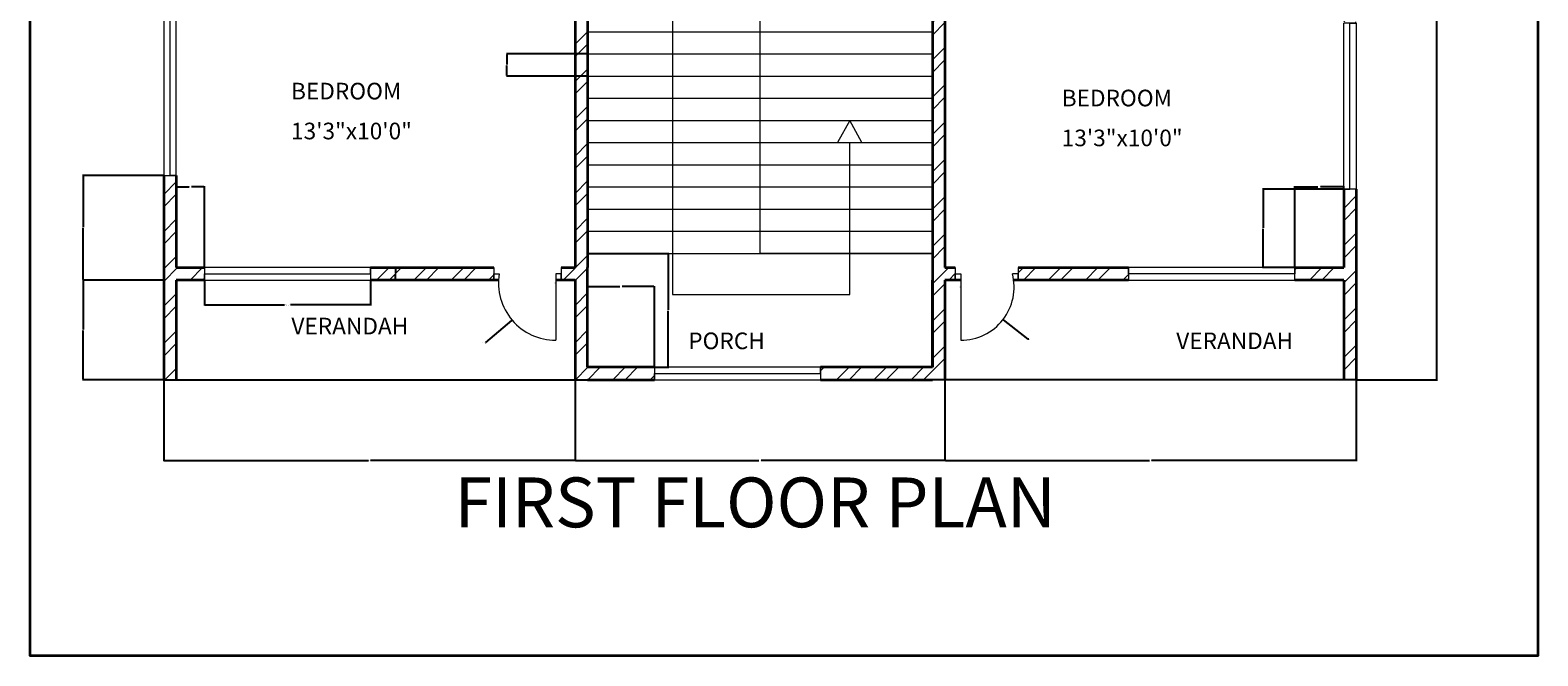
# Model space of a CAD drawing. Units: inches. Extents: x 2271 to 2815, y 1169 to 1838.
# Tile 1 of 4: x 2271 to 2815, y 1169 to 1395. Entities that reach past the tile are written whole.
import ezdxf

# ---------------------------------------------------------------- set-up
doc = ezdxf.new("R2010")
doc.units = ezdxf.units.IN
for name, color, linetype, lineweight in [('A-ANNO-DIMS', 2, 'Continuous', 18), ('A-ANNO-SYMB', 101, 'Continuous', 13), ('A-ANNO-TITL', 151, 'Continuous', 35), ('A-ANNO-TTLB', 7, 'Continuous', 35), ('A-AREA-IDEN', 7, 'Continuous', 18), ('A-DOOR', 11, 'Continuous', 18), ('A-FLOR-EDGE', 7, 'Continuous', 25), ('A-FLOR-STRS', 101, 'Continuous', 18), ('A-GLAZ', 181, 'Continuous', 18), ('A-WALL', 7, 'Continuous', 35)]:
    doc.layers.add(name, color=color, linetype=linetype, lineweight=lineweight)
doc.layers.add('A-WALL-PATT', color=9, linetype='Continuous', lineweight=13, true_color=0xafd9aa)
doc.styles.get("Standard").update_dxf_attribs({"font": 'arial.ttf'})
doc.dimstyles.get("Standard").update_dxf_attribs({"dimtxt": 0.18, "dimasz": 0.18, "dimexe": 0.18, "dimexo": 0.0625, "dimgap": 0.09, "dimtad": 0, "dimtih": 1, "dimtoh": 1, "dimdec": 4, "dimzin": 0, "dimdsep": 46, "dimtxsty": 'Standard', "dimcen": 0.09, "dimadec": 0, "dimazin": 0, "dimtfac": 1, "dimtdec": 4, "dimtofl": 0, "dimtmove": 0, "dimatfit": 3, "dimfxl": 1, "dimtolj": 1, "dimtzin": 0, "dimarcsym": 0})

# ---------------------------------------------------------------- blocks, each defined once
blk = doc.blocks.new('WIN-60IN')
for p, q in [((0, 4.5), (0, 0)), ((60, 4.5), (0, 4.5)), ((0, 0), (0, 2.25)), ((0, 2.25), (60, 2.25)), ((0, 0), (60, 0)), ((60, 2.25), (60, 4.5)), ((60, 4.5), (60, 0))]:
    blk.add_line(p, q)
blk = doc.blocks.new('*D3')
at = {"layer": 'A-ANNO-DIMS', "color": 0, "lineweight": -2, "transparency": 16777216}
for p, q in [((2333.47, 1304.47), (2333.47, 1295.35)), ((2393.47, 1304.47), (2393.47, 1295.35)), ((2333.65, 1295.53), (2362.35, 1295.53)), ((2393.29, 1295.53), (2364.58, 1295.53))]:
    blk.add_line(p, q, dxfattribs=at)
at = {"layer": 'A-ANNO-DIMS', "color": 0, "transparency": 16777216}
for points in [[(2333.65, 1295.56), (2333.65, 1295.5), (2333.47, 1295.53)], [(2393.29, 1295.56), (2393.29, 1295.5), (2393.47, 1295.53)]]:
    blk.add_solid(points, dxfattribs=at)
at = {"layer": 'Defpoints', "color": 0, "transparency": 16777216}
for p in [(2333.47, 1304.53), (2393.47, 1304.53), (2393.47, 1295.53)]:
    blk.add_point(p, dxfattribs=at)
at = {"layer": 'A-ANNO-DIMS', "color": 0, "transparency": 16777216, "insert": (2363.47, 1295.53), "char_height": 0.18, "attachment_point": 5}
blk.add_mtext('\\A1;WINDOW 60 TYP.', dxfattribs=at)
blk = doc.blocks.new('*D4')
at = {"layer": 'A-ANNO-DIMS', "color": 0, "lineweight": -2, "transparency": 16777216}
for p, q in [((2393.53, 1309.03), (2402.65, 1309.03)), ((2402.47, 1308.85), (2402.47, 1306.96)), ((2402.47, 1304.71), (2402.47, 1306.6)), ((2393.53, 1304.53), (2402.65, 1304.53))]:
    blk.add_line(p, q, dxfattribs=at)
at = {"layer": 'A-ANNO-DIMS', "color": 0, "transparency": 16777216}
for points in [[(2402.44, 1308.85), (2402.5, 1308.85), (2402.47, 1309.03)], [(2402.44, 1304.71), (2402.5, 1304.71), (2402.47, 1304.53)]]:
    blk.add_solid(points, dxfattribs=at)
at = {"layer": 'Defpoints', "color": 0, "transparency": 16777216}
for p in [(2393.47, 1309.03), (2402.47, 1309.03), (2393.47, 1304.53)]:
    blk.add_point(p, dxfattribs=at)
at = {"layer": 'A-ANNO-DIMS', "color": 0, "transparency": 16777216, "insert": (2402.47, 1306.78), "char_height": 0.18, "attachment_point": 5}
blk.add_mtext('\\A1;5 TYP.', dxfattribs=at)
blk = doc.blocks.new('*D8')
at = {"layer": 'A-ANNO-DIMS', "color": 0, "lineweight": -2, "transparency": 16777216}
for p, q in [((2749.36, 1787.53), (2778.63, 1787.53)), ((2778.45, 1787.35), (2778.45, 1528.21)), ((2778.45, 1268.71), (2778.45, 1527.85)), ((2749.36, 1268.53), (2778.63, 1268.53))]:
    blk.add_line(p, q, dxfattribs=at)
at = {"layer": 'A-ANNO-DIMS', "color": 0, "transparency": 16777216}
for points in [[(2778.42, 1787.35), (2778.48, 1787.35), (2778.45, 1787.53)], [(2778.42, 1268.71), (2778.48, 1268.71), (2778.45, 1268.53)]]:
    blk.add_solid(points, dxfattribs=at)
at = {"layer": 'Defpoints', "color": 0, "transparency": 16777216}
for p in [(2749.3, 1787.53), (2778.45, 1787.53), (2749.3, 1268.53)]:
    blk.add_point(p, dxfattribs=at)
at = {"layer": 'A-ANNO-DIMS', "color": 0, "transparency": 16777216, "insert": (2778.45, 1528.03), "char_height": 0.18, "attachment_point": 5}
blk.add_mtext('\\A1;519', dxfattribs=at)
blk = doc.blocks.new('*D9')
at = {"layer": 'A-ANNO-DIMS', "color": 0, "lineweight": -2, "transparency": 16777216}
for p, q in [((2318.8, 1268.47), (2318.8, 1239.2)), ((2467.3, 1268.47), (2467.3, 1239.2)), ((2318.98, 1239.38), (2392.66, 1239.38)), ((2467.12, 1239.38), (2393.44, 1239.38))]:
    blk.add_line(p, q, dxfattribs=at)
at = {"layer": 'A-ANNO-DIMS', "color": 0, "transparency": 16777216}
for points in [[(2318.98, 1239.41), (2318.98, 1239.35), (2318.8, 1239.38)], [(2467.12, 1239.41), (2467.12, 1239.35), (2467.3, 1239.38)]]:
    blk.add_solid(points, dxfattribs=at)
at = {"layer": 'Defpoints', "color": 0, "transparency": 16777216}
for p in [(2318.8, 1268.53), (2467.3, 1268.53), (2467.3, 1239.38)]:
    blk.add_point(p, dxfattribs=at)
at = {"layer": 'A-ANNO-DIMS', "color": 0, "transparency": 16777216, "insert": (2393.05, 1239.38), "char_height": 0.18, "attachment_point": 5}
blk.add_mtext('\\A1;148.5', dxfattribs=at)
blk = doc.blocks.new('*D10')
at = {"layer": 'A-ANNO-DIMS', "color": 0, "lineweight": -2, "transparency": 16777216}
for p, q in [((2467.3, 1268.47), (2467.3, 1239.2)), ((2600.8, 1268.47), (2600.8, 1239.2)), ((2467.48, 1239.38), (2533.66, 1239.38)), ((2600.62, 1239.38), (2534.44, 1239.38))]:
    blk.add_line(p, q, dxfattribs=at)
at = {"layer": 'A-ANNO-DIMS', "color": 0, "transparency": 16777216}
for points in [[(2467.48, 1239.41), (2467.48, 1239.35), (2467.3, 1239.38)], [(2600.62, 1239.41), (2600.62, 1239.35), (2600.8, 1239.38)]]:
    blk.add_solid(points, dxfattribs=at)
at = {"layer": 'Defpoints', "color": 0, "transparency": 16777216}
for p in [(2467.3, 1268.53), (2600.8, 1268.53), (2600.8, 1239.38)]:
    blk.add_point(p, dxfattribs=at)
at = {"layer": 'A-ANNO-DIMS', "color": 0, "transparency": 16777216, "insert": (2534.05, 1239.38), "char_height": 0.18, "attachment_point": 5}
blk.add_mtext('\\A1;133.5', dxfattribs=at)
blk = doc.blocks.new('*D11')
at = {"layer": 'A-ANNO-DIMS', "color": 0, "lineweight": -2, "transparency": 16777216}
for p, q in [((2600.8, 1268.47), (2600.8, 1239.2)), ((2749.3, 1268.47), (2749.3, 1239.2)), ((2600.98, 1239.38), (2674.66, 1239.38)), ((2749.12, 1239.38), (2675.44, 1239.38))]:
    blk.add_line(p, q, dxfattribs=at)
at = {"layer": 'A-ANNO-DIMS', "color": 0, "transparency": 16777216}
for points in [[(2600.98, 1239.41), (2600.98, 1239.35), (2600.8, 1239.38)], [(2749.12, 1239.41), (2749.12, 1239.35), (2749.3, 1239.38)]]:
    blk.add_solid(points, dxfattribs=at)
at = {"layer": 'Defpoints', "color": 0, "transparency": 16777216}
for p in [(2600.8, 1268.53), (2749.3, 1268.53), (2749.3, 1239.38)]:
    blk.add_point(p, dxfattribs=at)
at = {"layer": 'A-ANNO-DIMS', "color": 0, "transparency": 16777216, "insert": (2675.05, 1239.38), "char_height": 0.18, "attachment_point": 5}
blk.add_mtext('\\A1;148.5', dxfattribs=at)
blk = doc.blocks.new('*D12')
at = {"layer": 'A-ANNO-DIMS', "color": 0, "lineweight": -2, "transparency": 16777216}
for p, q in [((2318.74, 1304.53), (2289.47, 1304.53)), ((2289.65, 1304.35), (2289.65, 1286.71)), ((2289.65, 1268.71), (2289.65, 1286.35)), ((2318.74, 1268.53), (2289.47, 1268.53))]:
    blk.add_line(p, q, dxfattribs=at)
at = {"layer": 'A-ANNO-DIMS', "color": 0, "transparency": 16777216}
for points in [[(2289.62, 1304.35), (2289.68, 1304.35), (2289.65, 1304.53)], [(2289.62, 1268.71), (2289.68, 1268.71), (2289.65, 1268.53)]]:
    blk.add_solid(points, dxfattribs=at)
at = {"layer": 'Defpoints', "color": 0, "transparency": 16777216}
for p in [(2289.65, 1304.53), (2318.8, 1304.53), (2318.8, 1268.53)]:
    blk.add_point(p, dxfattribs=at)
at = {"layer": 'A-ANNO-DIMS', "color": 0, "transparency": 16777216, "insert": (2289.65, 1286.53), "char_height": 0.18, "attachment_point": 5}
blk.add_mtext('\\A1;36', dxfattribs=at)
blk = doc.blocks.new('*D13')
at = {"layer": 'A-ANNO-DIMS', "color": 0, "lineweight": -2, "transparency": 16777216}
for p, q in [((2318.74, 1342.31), (2289.47, 1342.31)), ((2289.65, 1342.13), (2289.65, 1323.6)), ((2289.65, 1304.71), (2289.65, 1323.24)), ((2318.74, 1304.53), (2289.47, 1304.53))]:
    blk.add_line(p, q, dxfattribs=at)
at = {"layer": 'A-ANNO-DIMS', "color": 0, "transparency": 16777216}
for points in [[(2289.62, 1342.13), (2289.68, 1342.13), (2289.65, 1342.31)], [(2289.62, 1304.71), (2289.68, 1304.71), (2289.65, 1304.53)]]:
    blk.add_solid(points, dxfattribs=at)
at = {"layer": 'Defpoints', "color": 0, "transparency": 16777216}
for p in [(2289.65, 1342.31), (2318.8, 1342.31), (2318.8, 1304.53)]:
    blk.add_point(p, dxfattribs=at)
at = {"layer": 'A-ANNO-DIMS', "color": 0, "transparency": 16777216, "insert": (2289.65, 1323.42), "char_height": 0.18, "attachment_point": 5}
blk.add_mtext('\\A1;37.78', dxfattribs=at)
blk = doc.blocks.new('*D24')
at = {"layer": 'A-ANNO-DIMS', "color": 0, "lineweight": -2, "transparency": 16777216}
for p, q in [((2471.86, 1314.17), (2501.13, 1314.17)), ((2500.95, 1313.99), (2500.95, 1293.78)), ((2500.95, 1273.21), (2500.95, 1293.42)), ((2471.86, 1273.03), (2501.13, 1273.03))]:
    blk.add_line(p, q, dxfattribs=at)
at = {"layer": 'A-ANNO-DIMS', "color": 0, "transparency": 16777216}
for points in [[(2500.92, 1313.99), (2500.98, 1313.99), (2500.95, 1314.17)], [(2500.92, 1273.21), (2500.98, 1273.21), (2500.95, 1273.03)]]:
    blk.add_solid(points, dxfattribs=at)
at = {"layer": 'Defpoints', "color": 0, "transparency": 16777216}
for p in [(2471.8, 1314.17), (2471.8, 1273.03), (2500.95, 1273.03)]:
    blk.add_point(p, dxfattribs=at)
at = {"layer": 'A-ANNO-DIMS', "color": 0, "transparency": 16777216, "insert": (2500.95, 1293.6), "char_height": 0.18, "attachment_point": 5}
blk.add_mtext('\\A1;41.14', dxfattribs=at)
blk = doc.blocks.new('*D25')
at = {"layer": 'A-ANNO-DIMS', "color": 0, "lineweight": -2, "transparency": 16777216}
for p, q in [((2471.74, 1386.17), (2442.47, 1386.17)), ((2442.65, 1385.99), (2442.65, 1382.35)), ((2471.74, 1378.17), (2442.47, 1378.17)), ((2442.65, 1378.35), (2442.65, 1381.99))]:
    blk.add_line(p, q, dxfattribs=at)
at = {"layer": 'A-ANNO-DIMS', "color": 0, "transparency": 16777216}
for points in [[(2442.62, 1385.99), (2442.68, 1385.99), (2442.65, 1386.17)], [(2442.62, 1378.35), (2442.68, 1378.35), (2442.65, 1378.17)]]:
    blk.add_solid(points, dxfattribs=at)
at = {"layer": 'Defpoints', "color": 0, "transparency": 16777216}
for p in [(2442.65, 1386.17), (2471.8, 1386.17), (2471.8, 1378.17)]:
    blk.add_point(p, dxfattribs=at)
at = {"layer": 'A-ANNO-DIMS', "color": 0, "transparency": 16777216, "insert": (2442.65, 1382.17), "char_height": 0.18, "attachment_point": 5}
blk.add_mtext('\\A1;8', dxfattribs=at)
blk = doc.blocks.new('*D30')
at = {"layer": 'A-ANNO-DIMS', "color": 0, "lineweight": -2, "transparency": 16777216}
for p, q in [((2323.3, 1309.09), (2323.3, 1338.36)), ((2323.48, 1338.18), (2327.93, 1338.18)), ((2333.29, 1338.18), (2328.84, 1338.18)), ((2333.47, 1309.09), (2333.47, 1338.36))]:
    blk.add_line(p, q, dxfattribs=at)
at = {"layer": 'A-ANNO-DIMS', "color": 0, "transparency": 16777216}
for points in [[(2323.48, 1338.21), (2323.48, 1338.15), (2323.3, 1338.18)], [(2333.29, 1338.21), (2333.29, 1338.15), (2333.47, 1338.18)]]:
    blk.add_solid(points, dxfattribs=at)
at = {"layer": 'Defpoints', "color": 0, "transparency": 16777216}
for p in [(2333.47, 1338.18), (2323.3, 1309.03), (2333.47, 1309.03)]:
    blk.add_point(p, dxfattribs=at)
at = {"layer": 'A-ANNO-DIMS', "color": 0, "transparency": 16777216, "insert": (2328.38, 1338.18), "char_height": 0.18, "attachment_point": 5}
blk.add_mtext('\\A1;10.166', dxfattribs=at)
blk = doc.blocks.new('*D31')
at = {"layer": 'A-ANNO-DIMS', "color": 0, "lineweight": -2, "transparency": 16777216}
for p, q in [((2727.09, 1309.09), (2727.09, 1338.36)), ((2727.27, 1338.18), (2735.49, 1338.18)), ((2744.62, 1338.18), (2736.4, 1338.18)), ((2744.8, 1309.09), (2744.8, 1338.36))]:
    blk.add_line(p, q, dxfattribs=at)
at = {"layer": 'A-ANNO-DIMS', "color": 0, "transparency": 16777216}
for points in [[(2727.27, 1338.21), (2727.27, 1338.15), (2727.09, 1338.18)], [(2744.62, 1338.21), (2744.62, 1338.15), (2744.8, 1338.18)]]:
    blk.add_solid(points, dxfattribs=at)
at = {"layer": 'Defpoints', "color": 0, "transparency": 16777216}
for p in [(2744.8, 1338.18), (2727.09, 1309.03), (2744.8, 1309.03)]:
    blk.add_point(p, dxfattribs=at)
at = {"layer": 'A-ANNO-DIMS', "color": 0, "transparency": 16777216, "insert": (2735.94, 1338.18), "char_height": 0.18, "attachment_point": 5}
blk.add_mtext('\\A1;17.714', dxfattribs=at)
blk = doc.blocks.new('*D32')
at = {"layer": 'A-ANNO-DIMS', "color": 0, "lineweight": -2, "transparency": 16777216}
for p, q in [((2471.8, 1273.09), (2471.8, 1302.36)), ((2471.98, 1302.18), (2483.47, 1302.18)), ((2495.74, 1302.18), (2484.25, 1302.18)), ((2495.92, 1273.09), (2495.92, 1302.36))]:
    blk.add_line(p, q, dxfattribs=at)
at = {"layer": 'A-ANNO-DIMS', "color": 0, "transparency": 16777216}
for points in [[(2471.98, 1302.21), (2471.98, 1302.15), (2471.8, 1302.18)], [(2495.74, 1302.21), (2495.74, 1302.15), (2495.92, 1302.18)]]:
    blk.add_solid(points, dxfattribs=at)
at = {"layer": 'Defpoints', "color": 0, "transparency": 16777216}
for p in [(2495.92, 1302.18), (2471.8, 1273.03), (2495.92, 1273.03)]:
    blk.add_point(p, dxfattribs=at)
at = {"layer": 'A-ANNO-DIMS', "color": 0, "transparency": 16777216, "insert": (2483.86, 1302.18), "char_height": 0.18, "attachment_point": 5}
blk.add_mtext('\\A1;24.12', dxfattribs=at)
blk = doc.blocks.new('*D33')
at = {"layer": 'A-ANNO-DIMS', "color": 0, "lineweight": -2, "transparency": 16777216}
for p, q in [((2744.74, 1337.31), (2715.47, 1337.31)), ((2715.65, 1337.13), (2715.65, 1323.35)), ((2715.65, 1309.21), (2715.65, 1322.99)), ((2744.74, 1309.03), (2715.47, 1309.03))]:
    blk.add_line(p, q, dxfattribs=at)
at = {"layer": 'A-ANNO-DIMS', "color": 0, "transparency": 16777216}
for points in [[(2715.62, 1337.13), (2715.68, 1337.13), (2715.65, 1337.31)], [(2715.62, 1309.21), (2715.68, 1309.21), (2715.65, 1309.03)]]:
    blk.add_solid(points, dxfattribs=at)
at = {"layer": 'Defpoints', "color": 0, "transparency": 16777216}
for p in [(2715.65, 1337.31), (2744.8, 1337.31), (2744.8, 1309.03)]:
    blk.add_point(p, dxfattribs=at)
at = {"layer": 'A-ANNO-DIMS', "color": 0, "transparency": 16777216, "insert": (2715.65, 1323.17), "char_height": 0.18, "attachment_point": 5}
blk.add_mtext('\\A1;28.28', dxfattribs=at)
blk = doc.blocks.new('*D43')
at = {"layer": 'A-ANNO-DIMS', "color": 0, "lineweight": -2, "transparency": 16777216}
for p, q in [((2460.23, 1303.47), (2460.41, 1303.47)), ((2460.32, 1303.38), (2460.32, 1303.56)), ((2435.11, 1282.02), (2444.43, 1289.95)), ((2434.93, 1282.02), (2435.11, 1282.02))]:
    blk.add_line(p, q, dxfattribs=at)
at = {"layer": 'A-ANNO-DIMS', "color": 0, "transparency": 16777216}
blk.add_solid([(2444.41, 1289.97), (2444.44, 1289.92), (2444.56, 1290.06)], dxfattribs=at)
at = {"layer": 'Defpoints', "color": 0, "transparency": 16777216}
for p in [(2460.32, 1303.47), (2444.56, 1290.06)]:
    blk.add_point(p, dxfattribs=at)
at = {"layer": 'A-ANNO-DIMS', "color": 0, "transparency": 16777216, "insert": (2434.38, 1282.02), "char_height": 0.18, "attachment_point": 5}
blk.add_mtext('\\A1;R20.692', dxfattribs=at)
blk = doc.blocks.new('*D45')
at = {"layer": 'A-ANNO-DIMS', "color": 0, "lineweight": -2, "transparency": 16777216}
for p, q in [((2606.47, 1302.02), (2606.65, 1302.02)), ((2606.56, 1301.93), (2606.56, 1302.11)), ((2630.87, 1283.14), (2621.9, 1290.11)), ((2631.05, 1283.14), (2630.87, 1283.14))]:
    blk.add_line(p, q, dxfattribs=at)
at = {"layer": 'A-ANNO-DIMS', "color": 0, "transparency": 16777216}
blk.add_solid([(2621.91, 1290.13), (2621.88, 1290.09), (2621.75, 1290.22)], dxfattribs=at)
at = {"layer": 'Defpoints', "color": 0, "transparency": 16777216}
for p in [(2606.56, 1302.02), (2621.75, 1290.22)]:
    blk.add_point(p, dxfattribs=at)
at = {"layer": 'A-ANNO-DIMS', "color": 0, "transparency": 16777216, "insert": (2631.53, 1283.14), "char_height": 0.18, "attachment_point": 5}
blk.add_mtext('\\A1;R19.24', dxfattribs=at)

msp = doc.modelspace()

# ---------------------------------------------------------------- hatches: boundary and pattern name
at = {"layer": 'A-WALL-PATT'}
h = msp.add_hatch(dxfattribs=at)
h.set_pattern_fill('ANSI32', color=256)
h.paths.add_polyline_path([(2441.4917, 1751.5314), (2397.0578, 1751.5314), (2397.0578, 1747.0314), (2441.4917, 1747.0314), (2441.4917, 1749.2814)])
h.paths.add_polyline_path([(2471.8006, 1787.5314), (2467.3006, 1787.5314), (2467.3006, 1783.0314), (2467.3006, 1751.5314), (2463.4131, 1751.5314), (2463.4131, 1747.0314), (2467.3006, 1747.0314), (2467.3006, 1615.0314), (2465.0606, 1615.0314), (2465.0606, 1610.5314), (2474.7192, 1610.5314), (2474.7192, 1612.7814), (2474.7192, 1615.0314), (2471.8006, 1615.0314), (2471.8006, 1747.0314), (2482.8275, 1747.0314), (2482.8275, 1749.2814), (2482.8275, 1751.5314), (2471.8006, 1751.5314)])
h.paths.add_polyline_path([(2549.5185, 1751.5314), (2506.8275, 1751.5314), (2506.8275, 1747.0314), (2531.8006, 1747.0314), (2531.8006, 1615.0314), (2496.0724, 1615.0314), (2496.0724, 1610.5314), (2531.8006, 1610.5314), (2531.8006, 1458.2548), (2528.7405, 1458.2548), (2528.7405, 1453.7548), (2539.7806, 1453.7548), (2539.7806, 1456.0048), (2539.7806, 1458.2548), (2536.3006, 1458.2548), (2536.3006, 1610.5314), (2573.267, 1610.5314), (2573.267, 1612.5736), (2573.267, 1612.7912), (2573.267, 1615.0314), (2536.3006, 1615.0314), (2536.3006, 1747.0314), (2549.5185, 1747.0314)])
h.paths.add_polyline_path([(2600.8006, 1787.5314), (2596.3006, 1787.5314), (2596.3006, 1747.0314), (2596.3006, 1615.0314), (2593.1473, 1615.0314), (2593.1473, 1610.5314), (2603.416, 1610.5314), (2603.416, 1612.7814), (2603.416, 1615.0314), (2600.8006, 1615.0314), (2600.8006, 1747.0314), (2603.7892, 1747.0314), (2603.7892, 1749.2814), (2603.7892, 1751.5314), (2600.8006, 1751.5314)])
h.paths.add_polyline_path([(2596.3006, 1751.5314), (2573.5185, 1751.5314), (2573.5185, 1747.0314), (2596.3006, 1747.0314)])
h.paths.add_polyline_path([(2648.9302, 1749.2814), (2648.9302, 1751.5314), (2624.6394, 1751.5314), (2624.6394, 1747.0314), (2648.9302, 1747.0314)])
h.paths.add_polyline_path([(2749.3006, 1751.5314), (2749.3006, 1787.5314), (2744.8006, 1787.5314), (2744.8006, 1751.5314), (2708.9302, 1751.5314), (2708.9302, 1747.0314), (2744.8006, 1747.0314), (2744.8006, 1715.8571), (2749.3006, 1715.8571)])
h.paths.add_polyline_path([(2337.0578, 1749.2814), (2337.0578, 1751.5314), (2323.3006, 1751.5314), (2323.3006, 1787.5314), (2318.8006, 1787.5314), (2318.8006, 1751.5314), (2318.8006, 1712.2179), (2323.3006, 1712.2179), (2323.3006, 1747.0314), (2337.0578, 1747.0314)])
h.paths.add_polyline_path([(2402.757, 1615.0314), (2323.3006, 1615.0314), (2323.3006, 1652.2179), (2318.8006, 1652.2179), (2318.8006, 1610.5314), (2323.3006, 1610.5314), (2342.8006, 1610.5314), (2342.8006, 1602.42), (2347.3006, 1602.42), (2347.3006, 1610.5314), (2402.757, 1610.5314)])
h.paths.add_polyline_path([(2430.8006, 1568.5314), (2430.8006, 1610.5314), (2434.8435, 1610.5314), (2434.8435, 1612.7814), (2434.8435, 1615.0314), (2422.3947, 1615.0314), (2422.3947, 1612.7814), (2422.3947, 1610.5314), (2426.3006, 1610.5314), (2426.3006, 1568.5314), (2347.3006, 1568.5314), (2347.3006, 1578.42), (2342.8006, 1578.42), (2342.8006, 1568.5314), (2318.8006, 1568.5314), (2318.8006, 1546.0693), (2322.7121, 1546.0693), (2323.3006, 1546.0693), (2323.3006, 1564.0314), (2342.8006, 1564.0314), (2347.3006, 1564.0314), (2430.8006, 1564.0314)])
h.paths.add_polyline_path([(2430.8006, 1480.0314), (2323.3006, 1480.0314), (2323.3006, 1498.0693), (2321.0506, 1498.0693), (2318.8006, 1498.0693), (2318.8006, 1475.5314), (2342.8006, 1475.5314), (2342.8006, 1466.8218), (2347.3006, 1466.8218), (2347.3006, 1475.5314), (2426.3006, 1475.5314), (2426.3006, 1458.0149), (2430.8006, 1458.0149), (2430.8006, 1475.5314)])
h.paths.add_polyline_path([(2435.9471, 1433.5314), (2430.8006, 1433.5314), (2430.8006, 1437.7896), (2426.3006, 1437.7896), (2426.3006, 1433.5314), (2347.3006, 1433.5314), (2347.3006, 1442.8218), (2342.8006, 1442.8218), (2342.8006, 1433.5314), (2318.8006, 1433.5314), (2318.8006, 1402.3145), (2323.3006, 1402.3145), (2323.3006, 1429.0314), (2342.8006, 1429.0314), (2347.3006, 1429.0314), (2435.9471, 1429.0314)])
h.paths.add_polyline_path([(2323.3006, 1342.3145), (2321.0506, 1342.3145), (2318.8006, 1342.3145), (2318.8006, 1304.5314), (2318.8006, 1268.5314), (2323.3006, 1268.5314), (2323.3006, 1304.5314), (2333.4662, 1304.5314), (2333.4662, 1306.7814), (2333.4662, 1309.0314), (2323.3006, 1309.0314)])
h.paths.add_polyline_path([(2437.8933, 1306.7814), (2437.8933, 1309.0314), (2393.4662, 1309.0314), (2393.4662, 1304.5314), (2437.8933, 1304.5314)])
h.paths.add_polyline_path([(2471.8006, 1453.7548), (2493.7895, 1453.7548), (2493.7895, 1456.0048), (2493.7895, 1458.2548), (2467.3006, 1458.2548), (2467.3006, 1433.5314), (2463.7134, 1433.5314), (2463.7134, 1431.2814), (2463.7134, 1429.0314), (2467.3006, 1429.0314), (2467.3006, 1309.0314), (2462.3197, 1309.0314), (2462.3197, 1304.5314), (2467.3006, 1304.5314), (2467.3006, 1268.5314), (2471.8006, 1268.5314), (2495.9201, 1268.5314), (2495.9201, 1270.7814), (2495.9201, 1273.0314), (2471.8006, 1273.0314), (2471.8006, 1309.0314)])
h.paths.add_polyline_path([(2600.8006, 1458.2548), (2570.4818, 1458.2548), (2570.4818, 1453.7548), (2596.3006, 1453.7548), (2596.3006, 1429.0314), (2596.3006, 1273.0314), (2555.9201, 1273.0314), (2555.9201, 1268.5314), (2596.3006, 1268.5314), (2600.8006, 1268.5314), (2600.8006, 1304.5314), (2604.5593, 1304.5314), (2604.5593, 1306.7814), (2604.5593, 1309.0314), (2600.8006, 1309.0314), (2600.8006, 1429.0314)])
h.paths.add_polyline_path([(2667.0861, 1309.0314), (2627.2, 1309.0314), (2627.2, 1304.5314), (2667.0861, 1304.5314)])
h.paths.add_polyline_path([(2749.3006, 1309.0314), (2749.3006, 1337.3095), (2744.8006, 1337.3095), (2744.8006, 1309.0314), (2727.0861, 1309.0314), (2727.0861, 1306.7814), (2727.0861, 1304.5314), (2744.8006, 1304.5314), (2744.8006, 1268.5314), (2749.3006, 1268.5314), (2749.3006, 1304.5314)])
h.paths.add_polyline_path([(2749.3006, 1433.5314), (2725.3006, 1433.5314), (2725.3006, 1442.7202), (2720.8006, 1442.7202), (2720.8006, 1433.5314), (2636.8006, 1433.5314), (2636.8006, 1437.8287), (2634.5506, 1437.8287), (2632.3006, 1437.8287), (2632.3006, 1433.5314), (2630.1129, 1433.5314), (2630.1129, 1429.0314), (2744.8006, 1429.0314), (2744.8006, 1397.3095), (2749.3006, 1397.3095)])
h.paths.add_polyline_path([(2749.3006, 1480.0314), (2749.3006, 1502.0415), (2744.8006, 1502.0415), (2744.8006, 1480.0314), (2720.8006, 1480.0314), (2632.3006, 1480.0314), (2632.3006, 1457.7851), (2636.8006, 1457.7851), (2636.8006, 1475.5314), (2720.8006, 1475.5314), (2720.8006, 1466.7202), (2725.3006, 1466.7202), (2725.3006, 1475.5314), (2749.3006, 1475.5314)])
h.paths.add_polyline_path([(2749.3006, 1568.5314), (2725.3006, 1568.5314), (2725.3006, 1578.9125), (2720.8006, 1578.9125), (2720.8006, 1568.5314), (2641.8006, 1568.5314), (2641.8006, 1610.5314), (2645.4823, 1610.5314), (2645.4823, 1612.7814), (2645.4823, 1615.0314), (2631.895, 1615.0314), (2631.895, 1610.5314), (2637.3006, 1610.5314), (2637.3006, 1568.5314), (2637.3006, 1564.0314), (2720.8006, 1564.0314), (2725.3006, 1564.0314), (2744.8006, 1564.0314), (2744.8006, 1550.0415), (2747.0506, 1550.0415), (2749.3006, 1550.0415)])
h.paths.add_polyline_path([(2749.3006, 1655.8571), (2744.8006, 1655.8571), (2744.8006, 1615.0314), (2668.3453, 1615.0314), (2668.3453, 1610.5314), (2720.8006, 1610.5314), (2720.8006, 1602.9125), (2725.3006, 1602.9125), (2725.3006, 1610.5314), (2749.3006, 1610.5314)])
h.paths.add_polyline_path([(2512.9815, 1676.2212), (2512.9815, 1716.3099), (2486.1477, 1716.3099), (2486.1477, 1676.2212)], flags=9)

# ---------------------------------------------------------------- linework, layer by layer
at = {"layer": 'A-ANNO-SYMB'}
for p, q in [((2502.512, 1425.1721), (2502.512, 1299.2714)), ((2566.5002, 1362.1711), (2562.0124, 1354.1711)), ((2570.8077, 1354.1711), (2566.5002, 1362.1711)), ((2562.0124, 1354.1711), (2570.8077, 1354.1711)), ((2566.5002, 1299.2714), (2566.5002, 1354.1711)), ((2502.512, 1299.2714), (2566.5002, 1299.2714))]:
    msp.add_line(p, q, dxfattribs=at)
at = {"layer": 'A-ANNO-TTLB'}
msp.add_lwpolyline([(2270.5512, 1838.2339), (2814.8691, 1838.2339), (2814.8691, 1168.8883), (2270.5512, 1168.8883)], close=True, dxfattribs=at)
at = {"layer": 'A-DOOR'}
for p, q in [((2437.8933, 1309.0314), (2437.8933, 1304.5314)), ((2437.8933, 1304.5314), (2437.8933, 1306.7814)), ((2437.8933, 1306.7814), (2439.8933, 1306.7814)), ((2462.3197, 1306.7814), (2460.3197, 1306.7814)), ((2460.3197, 1306.7814), (2460.3197, 1282.7814)), ((2462.3197, 1309.0314), (2462.3197, 1304.5314)), ((2462.3197, 1304.5314), (2462.3197, 1306.7814)), ((2604.5593, 1309.0314), (2604.5593, 1304.5314)), ((2604.5593, 1304.5314), (2604.5593, 1306.7814)), ((2604.5593, 1306.7814), (2606.5593, 1306.7814)), ((2606.5593, 1306.7814), (2606.5593, 1282.7814)), ((2627.2, 1306.7814), (2625.2, 1306.7814)), ((2627.2, 1309.0314), (2627.2, 1304.5314)), ((2627.2, 1304.5314), (2627.2, 1306.7814))]:
    msp.add_line(p, q, dxfattribs=at)
for centre, radius, start, end in [((2460.3197, 1303.4739), 20.6925, 170.802213, 270), ((2606.5593, 1302.0205), 19.2391, 270, 14.327324)]:
    msp.add_arc(centre, radius, start, end, dxfattribs=at)
at = {"layer": 'A-FLOR-EDGE'}
for p, q in [((2318.8006, 1268.5314), (2471.8006, 1268.5314)), ((2749.3006, 1268.5314), (2596.3006, 1268.5314))]:
    msp.add_line(p, q, dxfattribs=at)
at = {"layer": 'A-FLOR-STRS'}
for p, q in [((2534.0506, 1314.1711), (2534.0506, 1418.1711)), ((2471.8006, 1394.1711), (2596.3006, 1394.1711)), ((2471.8006, 1386.1711), (2596.3006, 1386.1711)), ((2471.8006, 1378.1711), (2596.3006, 1378.1711)), ((2471.8006, 1370.1711), (2596.3006, 1370.1711)), ((2471.8006, 1362.1711), (2596.3006, 1362.1711)), ((2471.8006, 1354.1711), (2596.3006, 1354.1711)), ((2471.8006, 1346.1711), (2596.3006, 1346.1711)), ((2471.8006, 1338.1711), (2596.3006, 1338.1711)), ((2471.8006, 1330.1711), (2596.3006, 1330.1711)), ((2471.8006, 1322.1711), (2596.3006, 1322.1711)), ((2471.8006, 1314.1711), (2596.3006, 1314.1711)), ((2596.3006, 1314.1711), (2534.0506, 1314.1711))]:
    msp.add_line(p, q, dxfattribs=at)
at = {"layer": 'A-GLAZ'}
for p, q in [((2667.0861, 1306.7814), (2667.0861, 1309.0314)), ((2667.0861, 1309.0314), (2667.0861, 1304.5314)), ((2727.0861, 1309.0314), (2667.0861, 1309.0314)), ((2727.0861, 1306.7814), (2667.0861, 1306.7814)), ((2727.0861, 1304.5314), (2727.0861, 1309.0314)), ((2727.0861, 1309.0314), (2727.0861, 1306.7814)), ((2667.0861, 1304.5314), (2727.0861, 1304.5314))]:
    msp.add_line(p, q, dxfattribs=at)
at = {"layer": 'A-WALL'}
for p, q in [((2471.8006, 1453.7548), (2471.8006, 1309.0314)), ((2467.3006, 1429.0314), (2467.3006, 1309.0314)), ((2596.3006, 1429.0314), (2596.3006, 1273.0314)), ((2600.8006, 1429.0314), (2600.8006, 1309.0314)), ((2318.8006, 1342.3145), (2318.8006, 1304.5314)), ((2323.3006, 1342.3145), (2323.3006, 1309.0314)), ((2323.3006, 1342.3145), (2323.3006, 1309.0314)), ((2744.8006, 1337.3095), (2744.8006, 1309.0314)), ((2749.3006, 1337.3095), (2749.3006, 1304.5314)), ((2323.3006, 1309.0314), (2333.4662, 1309.0314)), ((2393.4662, 1309.0314), (2437.8933, 1309.0314)), ((2462.3197, 1309.0314), (2467.3006, 1309.0314)), ((2471.8006, 1273.0314), (2471.8006, 1309.0314)), ((2600.8006, 1309.0314), (2604.5593, 1309.0314)), ((2627.2, 1309.0314), (2667.0861, 1309.0314)), ((2727.0861, 1309.0314), (2744.8006, 1309.0314)), ((2749.3006, 1309.0314), (2749.3006, 1304.5314)), ((2318.8006, 1304.5314), (2318.8006, 1268.5314)), ((2323.3006, 1304.5314), (2323.3006, 1268.5314)), ((2333.4662, 1304.5314), (2323.3006, 1304.5314)), ((2439.6543, 1304.5314), (2393.4662, 1304.5314)), ((2467.3006, 1304.5314), (2460.3197, 1304.5314)), ((2467.3006, 1304.5314), (2467.3006, 1268.5314)), ((2596.3006, 1273.0314), (2596.3006, 1304.5314)), ((2600.8006, 1304.5314), (2600.8006, 1268.5314)), ((2606.5593, 1304.5314), (2600.8006, 1304.5314)), ((2667.0861, 1304.5314), (2625.6338, 1304.5314)), ((2744.8006, 1304.5314), (2727.0861, 1304.5314)), ((2744.8006, 1304.5314), (2744.8006, 1268.5314)), ((2749.3006, 1304.5314), (2749.3006, 1268.5314)), ((2495.9201, 1273.0314), (2471.8006, 1273.0314)), ((2471.8006, 1268.5314), (2495.9201, 1268.5314)), ((2596.3006, 1273.0314), (2555.9201, 1273.0314)), ((2596.3006, 1273.0314), (2555.9201, 1273.0314)), ((2555.9201, 1268.5314), (2596.3006, 1268.5314))]:
    msp.add_line(p, q, dxfattribs=at)

# ---------------------------------------------------------------- block references
at = {"layer": 'A-GLAZ', "rotation": 90}
msp.add_blockref('WIN-60IN', (2323.301, 1342.3147), dxfattribs=at)
at = {"layer": 'A-GLAZ', "extrusion": (0, 0, -1), "zscale": -1, "rotation": 90}
msp.add_blockref('WIN-60IN', (-2744.8001, 1337.3097), dxfattribs=at)
at = {"layer": 'A-GLAZ'}
for p in [(2333.4664, 1304.531), (2495.9203, 1268.531)]:
    msp.add_blockref('WIN-60IN', p, dxfattribs=at)

# ---------------------------------------------------------------- texts
at = {"layer": 'A-ANNO-TITL', "insert": (2423.7258, 1233.2741), "char_height": 18, "attachment_point": 1}
msp.add_mtext_dynamic_manual_height_columns('FIRST FLOOR PLAN ', width=370.609688, gutter_width=12.5, heights=[0], dxfattribs=at)
at = {"layer": 'A-AREA-IDEN', "char_height": 6, "attachment_point": 1, "line_spacing_factor": 1.44}
for s, width, insert in [('BEDROOM\\P13\'3"x10\'0"', 157.43502, (2364.7337, 1375.7286)), ('BEDROOM\\P13\'3"x10\'0"', 157.43502, (2642.9735, 1373.2323)), ('VERANDAH', 202.405664, (2364.864, 1290.9144)), ('PORCH', 72.166667, (2508.1439, 1285.5906)), ('VERANDAH', 202.405664, (2684.3123, 1285.5913))]:
    msp.add_mtext_dynamic_manual_height_columns(s, width=width, gutter_width=12.5, heights=[0], dxfattribs=dict(at, insert=insert))

# ---------------------------------------------------------------- dimensions: what is measured, and where the dimension line sits
at = {"layer": 'A-ANNO-DIMS'}
for base, p1, p2, angle, override, picture, middle in [((2778.4506, 1787.5314), (2749.3006, 1268.5314), (2749.3006, 1787.5314), 90, {"dimdec": 0, "dimlfac": 1, "dimrnd": 0, "dimzin": 0, "dimdsep": 46, "dimlunit": 2}, '*D8', (2778.4506, 1528.0314)), ((2442.6506, 1386.1711), (2471.8006, 1378.1711), (2471.8006, 1386.1711), 90, {"dimdec": 0, "dimlfac": 1, "dimrnd": 0, "dimzin": 0, "dimdsep": 46, "dimlunit": 2}, '*D25', (2442.6506, 1382.1711)), ((2289.6506, 1342.3145), (2318.8006, 1304.5314), (2318.8006, 1342.3145), 90, {"dimdec": 2, "dimlfac": 1, "dimrnd": 0, "dimzin": 0, "dimdsep": 46, "dimlunit": 2}, '*D13', (2289.6506, 1323.423)), ((2715.6506, 1337.3095), (2744.8006, 1309.0314), (2744.8006, 1337.3095), 90, {"dimdec": 2, "dimlfac": 1, "dimrnd": 0, "dimzin": 0, "dimdsep": 46, "dimlunit": 2}, '*D33', (2715.6506, 1323.1705)), ((2500.9506, 1273.0314), (2471.8006, 1314.1711), (2471.8006, 1273.0314), 270, {"dimdec": 2, "dimlfac": 1, "dimrnd": 0, "dimzin": 0, "dimdsep": 46, "dimlunit": 2}, '*D24', (2500.9506, 1293.6013)), ((2289.6506, 1304.5314), (2318.8006, 1268.5314), (2318.8006, 1304.5314), 90, {"dimdec": 0, "dimlfac": 1, "dimrnd": 0, "dimzin": 0, "dimdsep": 46, "dimlunit": 2}, '*D12', (2289.6506, 1286.5314))]:
    dim = msp.add_linear_dim(base=base, p1=p1, p2=p2, angle=angle, dimstyle='Standard', override=override, dxfattribs=at)
    dim.commit()
    dim.dimension.update_dxf_attribs({"geometry": picture, "text_midpoint": middle})
for base, p1, p2, override, picture, middle in [((2333.4662, 1338.1814), (2323.3006, 1309.0314), (2333.4662, 1309.0314), {"dimdec": 3, "dimlfac": 1, "dimrnd": 0, "dimzin": 0, "dimdsep": 46, "dimlunit": 2}, '*D30', (2328.3834, 1338.1814)), ((2744.80056, 1338.18142), (2727.08613, 1309.03142), (2744.80056, 1309.03142), {"dimdec": 3, "dimlfac": 1, "dimrnd": 0, "dimzin": 0, "dimdsep": 46, "dimlunit": 2}, '*D31', (2735.94335, 1338.18142)), ((2495.9201, 1302.1814), (2471.8006, 1273.0314), (2495.9201, 1273.0314), {"dimdec": 2, "dimlfac": 1, "dimrnd": 0, "dimzin": 0, "dimdsep": 46, "dimlunit": 2}, '*D32', (2483.8603, 1302.1814)), ((2467.3006, 1239.3814), (2318.8006, 1268.5314), (2467.3006, 1268.5314), {"dimdec": 1, "dimlfac": 1, "dimrnd": 0, "dimzin": 0, "dimdsep": 46, "dimlunit": 2}, '*D9', (2393.0506, 1239.3814)), ((2600.8006, 1239.3814), (2467.3006, 1268.5314), (2600.8006, 1268.5314), {"dimdec": 1, "dimlfac": 1, "dimrnd": 0, "dimzin": 0, "dimdsep": 46, "dimlunit": 2}, '*D10', (2534.0506, 1239.3814)), ((2749.3006, 1239.3814), (2600.8006, 1268.5314), (2749.3006, 1268.5314), {"dimdec": 1, "dimlfac": 1, "dimrnd": 0, "dimzin": 0, "dimdsep": 46, "dimlunit": 2}, '*D11', (2675.0506, 1239.3814))]:
    dim = msp.add_linear_dim(base=base, p1=p1, p2=p2, dimstyle='Standard', override=override, dxfattribs=at)
    dim.commit()
    dim.dimension.update_dxf_attribs({"geometry": picture, "text_midpoint": middle})
dim = msp.add_linear_dim(base=(2402.4661930743, 1309.0314174086), p1=(2393.4661930743, 1304.5314174086), p2=(2393.4661930743, 1309.0314174086), angle=90, text='<> TYP.', dimstyle='Standard', override={"dimdec": 0, "dimlfac": 1, "dimrnd": 0, "dimzin": 0, "dimdsep": 46, "dimlunit": 2}, dxfattribs=at)
dim.commit()
dim.dimension.update_dxf_attribs({"geometry": '*D4', "text_midpoint": (2402.4661930743, 1306.7814174086)})
dim = msp.add_linear_dim(base=(2393.4662, 1295.5314), p1=(2333.4662, 1304.5314), p2=(2393.4662, 1304.5314), text='WINDOW <> TYP.', dimstyle='Standard', override={"dimdec": 0, "dimlfac": 1, "dimrnd": 0, "dimzin": 0, "dimdsep": 46, "dimlunit": 2}, dxfattribs=at)
dim.commit()
dim.dimension.update_dxf_attribs({"geometry": '*D3', "text_midpoint": (2363.4662, 1295.5314)})
for center, mpoint, override, picture, middle in [((2460.3197, 1303.4739), (2444.5621, 1290.0621), {"dimdec": 3, "dimlfac": 1, "dimrnd": 0, "dimzin": 0, "dimdsep": 46, "dimlunit": 2}, '*D43', (2434.3787, 1282.015)), ((2606.5593, 1302.0205), (2621.7538, 1290.2192), {"dimdec": 2, "dimlfac": 1, "dimrnd": 0, "dimzin": 0, "dimdsep": 46, "dimlunit": 2}, '*D45', (2631.5299, 1283.1384))]:
    dim = msp.add_radius_dim(center=center, mpoint=mpoint, dimstyle='Standard', override=override, dxfattribs=at)
    dim.commit()
    dim.dimension.update_dxf_attribs({"geometry": picture, "text_midpoint": middle, "dimtype": 164})

doc.saveas('drawing.dxf')
